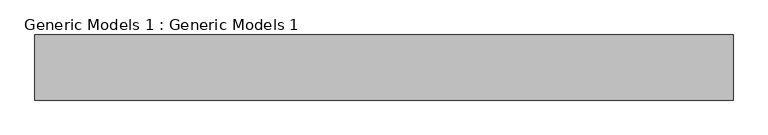
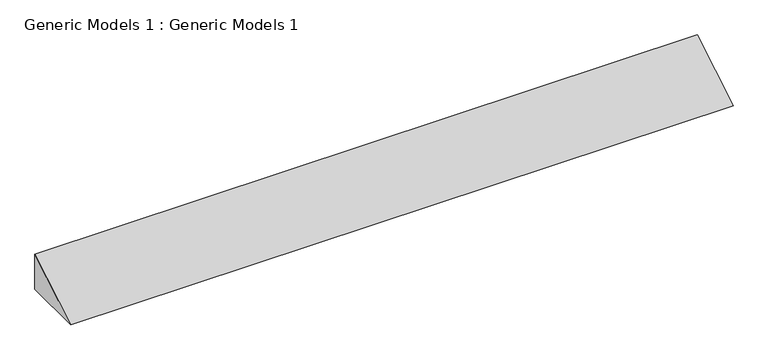
"""IFC4 building model written with IfcOpenShell, lengths in millimetres: proxy geometry, Generic Models 1 : Generic Models 1."""

from ifc_helpers import new_model, si_unit, frame, origin, place, context, project, spatial, polyline, outline, extrude, source, transform, mapped, element, save


def generic_models_1_generic_models_1_2c9bbbb1(model_context):
    return source(origin(), model_context, "Body", "SweptSolid", [
        extrude(outline(polyline([(-12412.3889249, 122.0948778), (-12412.3889249, -304.8), (-13122.8613112, -304.8), (-12412.3889249, 122.0948778)])), frame((-53238.4015344, 0.0, 0.0), z_axis=(1.0, 0.0, 0.0), x_axis=(0.0, 1.0, 0.0)), (0.0, 0.0, 1.0), 7612.6438535),
    ])


if __name__ == "__main__":
    model = new_model("IFC4")
    model_context = context("Model", 3, world=origin())
    ifc_project = project(units=[si_unit("LENGTHUNIT", "METRE", prefix="MILLI")], contexts=[model_context])
    site = spatial("IfcSite", under=ifc_project)
    building = spatial("IfcBuilding", under=site)
    placement = place(None, origin())
    generic_models_1_generic_models_1_shape = generic_models_1_generic_models_1_2c9bbbb1(model_context)
    element("IfcBuildingElementProxy", 1, Name="Generic Models 1 : Generic Models 1", ObjectType="Generic Models 1 : Generic Models 1", at=placement, inside=building, context=model_context, shape_type="MappedRepresentation", body=[
        mapped(generic_models_1_generic_models_1_shape, transform((0.0, 0.0, 0.0), x_axis=(1.0, 0.0, 0.0), y_axis=(0.0, 1.0, 0.0), z_axis=(0.0, 0.0, 1.0))),
    ])
    save(model, "model.ifc")

# Revit data of these elements
# Element 1 (IfcBuildingElementProxy, "Generic Models 1 : Generic Models 1")
#   Materials on its faces: "DARK WALNUT COLOUR"
# Materials
#   "DARK WALNUT COLOUR": class "Generic", colour RGB 120 120 120, transparency 0, Cost = 0
